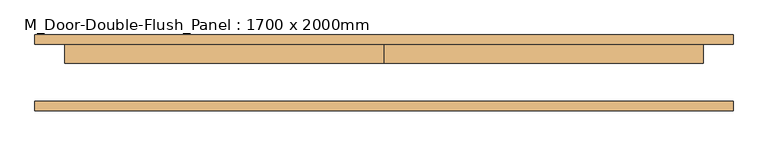
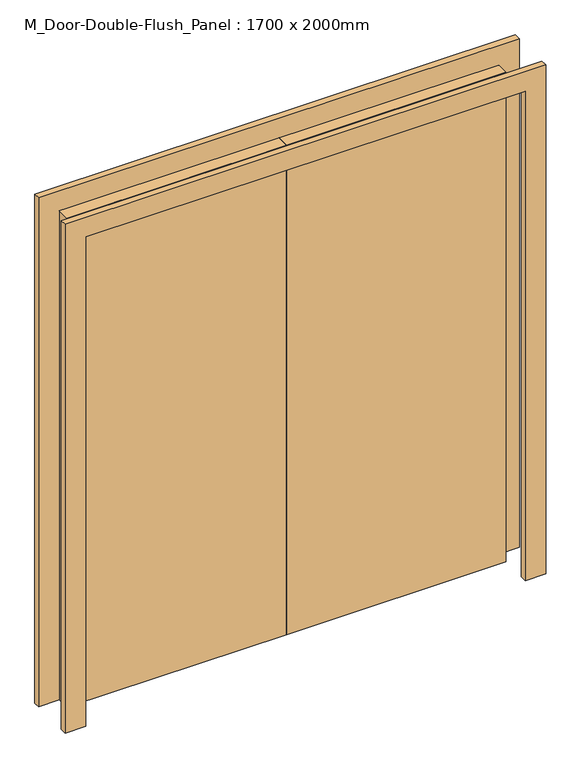
"""IFC4 building model written with IfcOpenShell, lengths in millimetres: door geometry, M_Door-Double-Flush_Panel : 1700 x 2000mm."""

from ifc_helpers import new_model, si_unit, frame, origin, origin_with_axes, place, context, project, spatial, polyline, outline, extrude, source, transform, mapped, element, save


def m_door_double_flush_panel_1700_x_2000mm_b668bbd0(model_context):
    return source(origin(), model_context, "Body", "SweptSolid", [
        extrude(outline(polyline([(2000.0, -850.0), (2000.0, 850.0), (0.0, 850.0), (0.0, 930.0), (2080.0, 930.0), (2080.0, -930.0), (0.0, -930.0), (0.0, -850.0), (2000.0, -850.0)])), frame((0.0, -101.2, 0.0), z_axis=(0.0, 1.0, 0.0), x_axis=(0.0, 0.0, 1.0)), (0.0, 0.0, 1.0), 25.0),
        extrude(outline(polyline([(2000.0, -850.0), (2000.0, 850.0), (0.0, 850.0), (0.0, 930.0), (2080.0, 930.0), (2080.0, -930.0), (0.0, -930.0), (0.0, -850.0), (2000.0, -850.0)])), frame((0.0, 76.2, 0.0), z_axis=(0.0, 1.0, 0.0), x_axis=(0.0, 0.0, 1.0)), (0.0, 0.0, 1.0), 25.0),
        extrude(outline(polyline([(0.0, 76.2), (850.0, 76.2), (850.0, 26.2), (0.0, 26.2), (0.0, 76.2)])), origin_with_axes(), (0.0, 0.0, 1.0), 2000.0),
        extrude(outline(polyline([(-850.0, 76.2), (0.0, 76.2), (0.0, 26.2), (-850.0, 26.2), (-850.0, 76.2)])), origin_with_axes(), (0.0, 0.0, 1.0), 2000.0),
    ])


if __name__ == "__main__":
    model = new_model("IFC4")
    model_context = context("Model", 3, world=origin())
    ifc_project = project(units=[si_unit("LENGTHUNIT", "METRE", prefix="MILLI")], contexts=[model_context])
    site = spatial("IfcSite", under=ifc_project)
    building = spatial("IfcBuilding", under=site)
    placement = place(None, origin())
    m_door_double_flush_panel_1700_x_2000mm_shape = m_door_double_flush_panel_1700_x_2000mm_b668bbd0(model_context)
    element("IfcDoor", 1, ObjectType="M_Door-Double-Flush_Panel : 1700 x 2000mm", at=placement, inside=building, context=model_context, shape_type="MappedRepresentation", body=[
        mapped(m_door_double_flush_panel_1700_x_2000mm_shape, transform((0.0, 0.0, 0.0), x_axis=(1.0, 0.0, 0.0), y_axis=(0.0, 1.0, 0.0), z_axis=(0.0, 0.0, 1.0))),
    ])
    save(model, "model.ifc")

# Revit data of these elements
# Type "M_Door-Double-Flush_Panel : 1700 x 2000mm"
#   Type Mark = "8"
#   Construction Type Id = "DOOR"
#   Assembly Code = "C1020"
#   Analytic Construction = "Wooden"
#   Thickness = 0' - 1.9685"
#   Thermal Resistance (R) = 2.5876 (h·ft²·°F)/BTU
#   Swing Angle [instance default] = 90.00°
#   Panel Width = 2' - 9.46457"
#   Heat Transfer Coefficient (U) = 0.3865 BTU/(h·ft²·°F)
#   Height = 6' - 6.74016"
#   Trim Projection Ext = 0' - 0.98425"
#   Trim Projection Int = 0' - 0.98425"
#   Trim Width = 0' - 3.14961"
#   Width = 5' - 6.92913"
#   Define Thermal Properties by = 1
#   Panel Material = Wood - Birch - Solid Stained Light Low Gloss
#   Trim Material = Paint - Sienna
#   Visual Light Transmittance = 0
#   Solar Heat Gain Coefficient = 0
#   Function = (empty or 0)
#   Wall Closure = (empty or 0)
# Element 1 (IfcDoor, "M_Door-Double-Flush_Panel : 1700 x 2000mm")
#   Materials on its faces: "Paint - Sienna", "Wood - Birch - Solid Stained Light Low Gloss"
# Materials
#   "Wood - Birch - Solid Stained Light Low Gloss": class "Wood", colour RGB 210 159 95, transparency 0, Cost = 0
#   "Paint - Sienna": colour RGB 118 70 51, transparency 0, Cost = 0
